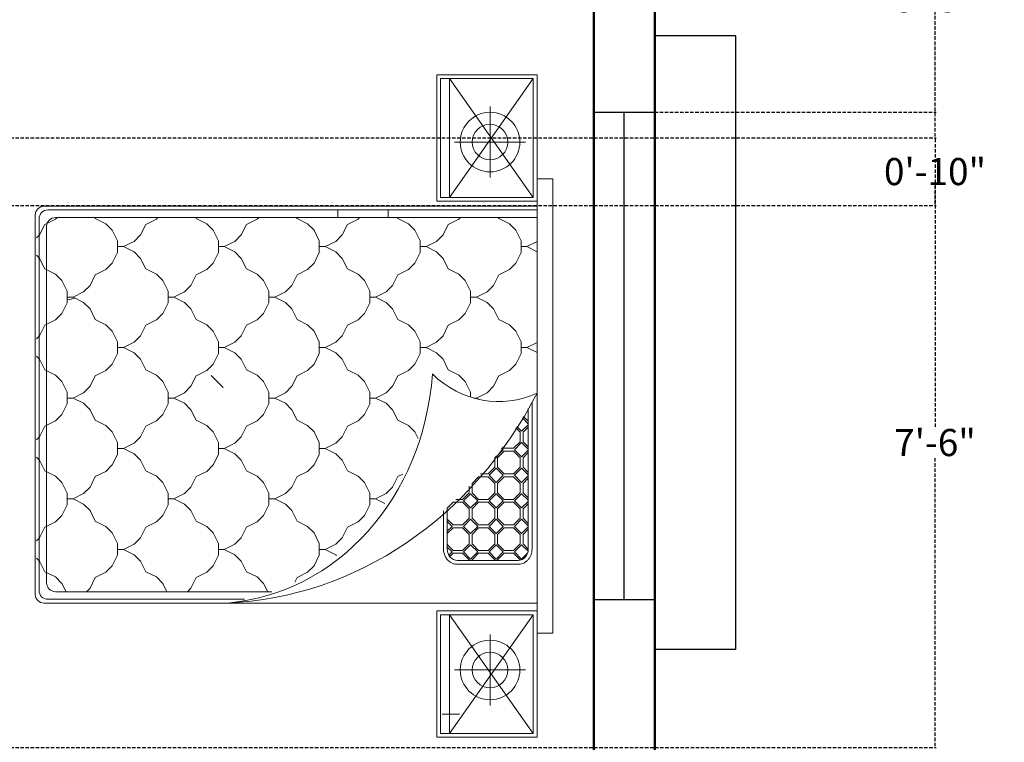
# Model space of a CAD drawing. Units: inches. Extents: x 513 to 1142, y 396 to 927.
# Tile 13 of 31: x 996 to 1142, y 507 to 614. Entities that reach past the tile are written whole.
import ezdxf

# ---------------------------------------------------------------- set-up
doc = ezdxf.new("R2010")
doc.units = ezdxf.units.IN
doc.header["$MEASUREMENT"] = 0
doc.linetypes.add('DASHED', pattern=[0.75, 0.5, -0.25])
for name, color, linetype, lineweight in [('A-ANNO-DIMS', 2, 'DASHED', 18), ('A-WALL', 7, 'Continuous', 50), ('furniture', 92, 'Continuous', 18), ('windows', 172, 'Continuous', 25)]:
    doc.layers.add(name, color=color, linetype=linetype, lineweight=lineweight)
doc.styles.get("Standard").update_dxf_attribs({"font": 'arial.ttf'})
doc.dimstyles.get("Standard").update_dxf_attribs({"dimtxt": 4, "dimasz": 0.18, "dimexe": 0.18, "dimexo": 0.0625, "dimgap": 0.09, "dimtad": 0, "dimtih": 1, "dimtoh": 1, "dimdec": 0, "dimrnd": 6, "dimzin": 0, "dimdsep": 46, "dimlunit": 3, "dimtxsty": 'Standard', "dimcen": 0.09, "dimadec": 0, "dimazin": 0, "dimtfac": 1, "dimtdec": 0, "dimtofl": 0, "dimtmove": 0, "dimatfit": 3, "dimfxl": 1, "dimtolj": 1, "dimtzin": 0, "dimarcsym": 0})

# ---------------------------------------------------------------- blocks, each defined once
blk = doc.blocks.new('A$C029D5C69')
for p, q in [((0.4164, 2.0693), (0.4164, 2.0066)), ((2.2315, 2.0693), (0.4164, 2.0693)), ((2.2315, 2.0066), (2.2315, 2.0693)), ((2.1114, 2.0087), (2.1114, 0.0351)), ((0, 1.606), (0, 2.0066)), ((0, 2.0066), (0.505, 2.0066)), ((0.0151, 1.6211), (0.0151, 1.9915)), ((0.0151, 1.9915), (0.4899, 1.9915)), ((0.4164, 2.0066), (2.2315, 2.0066)), ((0.4899, 1.9915), (0.4899, 1.6211)), ((0.505, 2.0066), (0.505, 1.606)), ((0.5252, 0.0351), (0.5252, 2.0066)), ((0.5403, 0.0502), (0.5403, 2.0066)), ((0.5706, 0.0805), (0.5706, 2.0066)), ((0.6869, 1.966), (0.6666, 2.0066)), ((0.7072, 2.0066), (0.6869, 1.966)), ((1.0902, 1.966), (1.0699, 2.0066)), ((1.1106, 2.0066), (1.0902, 1.966)), ((1.8954, 1.9865), (1.3081, 1.9865)), ((1.8954, 1.9713), (1.3339, 1.9713)), ((1.3849, 1.9713), (1.3656, 1.952)), ((1.3945, 1.9713), (1.3714, 1.9483)), ((1.4249, 1.945), (1.3986, 1.9713)), ((1.4288, 1.9507), (1.4081, 1.9713)), ((1.487, 1.9713), (1.4664, 1.9507)), ((1.4966, 1.9713), (1.4703, 1.945)), ((1.527, 1.945), (1.5007, 1.9713)), ((1.5309, 1.9507), (1.5102, 1.9713)), ((1.5891, 1.9713), (1.5685, 1.9507)), ((1.5987, 1.9713), (1.5724, 1.945)), ((1.6291, 1.945), (1.6028, 1.9713)), ((1.633, 1.9507), (1.6123, 1.9713)), ((1.6912, 1.9713), (1.6706, 1.9507)), ((1.7008, 1.9713), (1.6745, 1.945)), ((1.7312, 1.945), (1.7049, 1.9713)), ((1.7351, 1.9507), (1.7144, 1.9713)), ((1.7933, 1.9713), (1.7727, 1.9507)), ((1.8029, 1.9713), (1.7766, 1.945)), ((1.8333, 1.945), (1.807, 1.9713)), ((1.8372, 1.9507), (1.8165, 1.9713)), ((1.8954, 1.9713), (1.8748, 1.9507)), ((1.9043, 1.9707), (1.8787, 1.945)), ((1.9354, 1.945), (1.9114, 1.969)), ((2.6479, 2.0066), (2.1429, 2.0066)), ((2.1429, 2.0066), (2.1429, 1.606)), ((2.6328, 1.9915), (2.158, 1.9915)), ((2.158, 1.9915), (2.158, 1.6211)), ((2.6328, 1.6211), (2.6328, 1.9915)), ((2.6479, 1.606), (2.6479, 2.0066)), ((0.2689, 1.9609), (0.2689, 1.6764)), ((0.6634, 1.9425), (0.621, 1.9213)), ((0.6634, 1.9425), (0.621, 1.9213)), ((0.6869, 1.9425), (0.6634, 1.9425)), ((0.6869, 1.9425), (0.6869, 1.966)), ((0.6869, 1.9425), (0.6869, 1.966)), ((0.6869, 1.9425), (0.7104, 1.9425)), ((0.7528, 1.9213), (0.7104, 1.9425)), ((0.7528, 1.9213), (0.7104, 1.9425)), ((1.0668, 1.9425), (1.0244, 1.9213)), ((1.0668, 1.9425), (1.0244, 1.9213)), ((1.0902, 1.9425), (1.0668, 1.9425)), ((1.0902, 1.9425), (1.0902, 1.966)), ((1.0902, 1.9425), (1.0902, 1.966)), ((1.0902, 1.9425), (1.1137, 1.9425)), ((1.1561, 1.9213), (1.1137, 1.9425)), ((1.1561, 1.9213), (1.1137, 1.9425)), ((1.4249, 1.945), (1.4059, 1.926)), ((1.4288, 1.9394), (1.4116, 1.9222)), ((1.4476, 1.9507), (1.4288, 1.9507)), ((1.4288, 1.9393), (1.4476, 1.9393)), ((1.4476, 1.9507), (1.4664, 1.9507)), ((1.4664, 1.9393), (1.4476, 1.9393)), ((1.493, 1.9128), (1.4664, 1.9394)), ((1.4986, 1.9167), (1.4703, 1.945)), ((1.527, 1.945), (1.4986, 1.9167)), ((1.5309, 1.9394), (1.5043, 1.9128)), ((1.5497, 1.9507), (1.5309, 1.9507)), ((1.5309, 1.9393), (1.5497, 1.9393)), ((1.5497, 1.9507), (1.5685, 1.9507)), ((1.5685, 1.9393), (1.5497, 1.9393)), ((1.595, 1.9128), (1.5685, 1.9394)), ((1.6007, 1.9167), (1.5724, 1.945)), ((1.6291, 1.945), (1.6007, 1.9167)), ((1.633, 1.9394), (1.6064, 1.9128)), ((1.6518, 1.9507), (1.633, 1.9507)), ((1.633, 1.9393), (1.6518, 1.9393)), ((1.6518, 1.9507), (1.6706, 1.9507)), ((1.6706, 1.9393), (1.6518, 1.9393)), ((1.6971, 1.9128), (1.6706, 1.9394)), ((1.7028, 1.9167), (1.6745, 1.945)), ((1.7312, 1.945), (1.7028, 1.9167)), ((1.7351, 1.9394), (1.7085, 1.9128)), ((1.7539, 1.9507), (1.7351, 1.9507)), ((1.7351, 1.9393), (1.7539, 1.9393)), ((1.7539, 1.9507), (1.7727, 1.9507)), ((1.7727, 1.9393), (1.7539, 1.9393)), ((1.7992, 1.9128), (1.7727, 1.9394)), ((1.8049, 1.9167), (1.7766, 1.945)), ((1.8333, 1.945), (1.8049, 1.9167)), ((1.8372, 1.9394), (1.8106, 1.9128)), ((1.856, 1.9507), (1.8372, 1.9507)), ((1.8372, 1.9393), (1.856, 1.9393)), ((1.856, 1.9507), (1.8748, 1.9507)), ((1.8748, 1.9393), (1.856, 1.9393)), ((1.9013, 1.9128), (1.8748, 1.9394)), ((1.907, 1.9167), (1.8787, 1.945)), ((1.9354, 1.945), (1.907, 1.9167)), ((1.9393, 1.9394), (1.9127, 1.9128)), ((1.9393, 1.9393), (1.9404, 1.9393)), ((1.9414, 1.688), (1.9414, 1.931)), ((1.9565, 1.688), (1.9565, 1.931)), ((2.379, 1.9609), (2.379, 1.6764)), ((0.5955, 1.8958), (0.5743, 1.8534)), ((0.621, 1.9213), (0.5955, 1.8958)), ((0.7783, 1.8958), (0.7528, 1.9213)), ((0.7995, 1.8534), (0.7783, 1.8958)), ((0.9989, 1.8958), (0.9777, 1.8534)), ((1.0243, 1.9213), (0.9988, 1.8958)), ((1.1816, 1.8958), (1.1561, 1.9213)), ((1.2028, 1.8534), (1.1816, 1.8958)), ((1.493, 1.8752), (1.493, 1.9128)), ((1.5043, 1.8752), (1.5043, 1.9128)), ((1.595, 1.8752), (1.595, 1.9128)), ((1.6064, 1.8752), (1.6064, 1.9128)), ((1.6971, 1.8752), (1.6971, 1.9128)), ((1.7085, 1.8752), (1.7085, 1.9128)), ((1.7992, 1.8752), (1.7992, 1.9128)), ((1.8106, 1.8752), (1.8106, 1.9128)), ((1.9013, 1.8752), (1.9013, 1.9128)), ((1.9127, 1.8752), (1.9127, 1.9128)), ((0.5743, 1.8534), (0.5706, 1.8515)), ((0.5743, 1.8534), (0.5706, 1.8515)), ((0.8419, 1.8322), (0.7995, 1.8534)), ((0.8419, 1.8322), (0.7995, 1.8534)), ((0.9777, 1.8534), (0.9353, 1.8322)), ((0.9777, 1.8534), (0.9353, 1.8322)), ((1.2452, 1.8322), (1.2028, 1.8534)), ((1.2452, 1.8322), (1.2028, 1.8534)), ((1.493, 1.8752), (1.4867, 1.869)), ((1.4986, 1.8713), (1.4922, 1.8648)), ((1.527, 1.8429), (1.4986, 1.8713)), ((1.5309, 1.8486), (1.5043, 1.8752)), ((1.595, 1.8752), (1.5685, 1.8486)), ((1.6007, 1.8713), (1.5724, 1.8429)), ((1.6291, 1.8429), (1.6007, 1.8713)), ((1.633, 1.8486), (1.6064, 1.8752)), ((1.6971, 1.8752), (1.6706, 1.8486)), ((1.7028, 1.8713), (1.6745, 1.8429)), ((1.7312, 1.8429), (1.7028, 1.8713)), ((1.7351, 1.8486), (1.7085, 1.8752)), ((1.7992, 1.8752), (1.7727, 1.8486)), ((1.8049, 1.8713), (1.7766, 1.8429)), ((1.8333, 1.8429), (1.8049, 1.8713)), ((1.8372, 1.8486), (1.8106, 1.8752)), ((1.9013, 1.8752), (1.8748, 1.8486)), ((1.907, 1.8713), (1.8787, 1.8429)), ((1.9354, 1.8429), (1.907, 1.8713)), ((1.9393, 1.8486), (1.9127, 1.8752)), ((0.1267, 1.8186), (0.4111, 1.8186)), ((0.8674, 1.8067), (0.8419, 1.8322)), ((0.9352, 1.8322), (0.9097, 1.8067)), ((1.2707, 1.8067), (1.2452, 1.8322)), ((1.527, 1.8429), (1.5242, 1.8401)), ((1.5309, 1.8373), (1.5295, 1.8359)), ((1.5497, 1.8486), (1.5309, 1.8486)), ((1.5309, 1.8373), (1.5497, 1.8373)), ((1.5497, 1.8486), (1.5685, 1.8486)), ((1.5685, 1.8373), (1.5497, 1.8373)), ((1.595, 1.8107), (1.5685, 1.8373)), ((1.6007, 1.8146), (1.5724, 1.8429)), ((1.6291, 1.8429), (1.6007, 1.8146)), ((1.633, 1.8373), (1.6064, 1.8107)), ((1.6518, 1.8486), (1.633, 1.8486)), ((1.633, 1.8373), (1.6518, 1.8373)), ((1.6518, 1.8486), (1.6706, 1.8486)), ((1.6706, 1.8373), (1.6518, 1.8373)), ((1.6971, 1.8107), (1.6706, 1.8373)), ((1.7028, 1.8146), (1.6745, 1.8429)), ((1.7312, 1.8429), (1.7028, 1.8146)), ((1.7351, 1.8373), (1.7085, 1.8107)), ((1.7539, 1.8486), (1.7351, 1.8486)), ((1.7351, 1.8373), (1.7539, 1.8373)), ((1.7539, 1.8486), (1.7727, 1.8486)), ((1.7727, 1.8373), (1.7539, 1.8373)), ((1.7992, 1.8107), (1.7727, 1.8373)), ((1.8049, 1.8146), (1.7766, 1.8429)), ((1.8333, 1.8429), (1.8049, 1.8146)), ((1.8372, 1.8373), (1.8106, 1.8107)), ((1.856, 1.8486), (1.8372, 1.8486)), ((1.8372, 1.8373), (1.856, 1.8373)), ((1.856, 1.8486), (1.8748, 1.8486)), ((1.8748, 1.8373), (1.856, 1.8373)), ((1.9013, 1.8107), (1.8748, 1.8373)), ((1.907, 1.8146), (1.8787, 1.8429)), ((1.9354, 1.8429), (1.907, 1.8146)), ((1.9393, 1.8373), (1.9127, 1.8107)), ((1.9414, 1.8486), (1.9393, 1.8486)), ((1.9393, 1.8373), (1.9414, 1.8373)), ((2.2367, 1.8186), (2.5212, 1.8186)), ((0.8886, 1.7643), (0.8674, 1.8067)), ((0.9098, 1.8067), (0.8886, 1.7643)), ((1.2919, 1.7643), (1.2707, 1.8067)), ((1.2981, 1.7768), (1.2919, 1.7643)), ((1.595, 1.7806), (1.595, 1.8107)), ((1.6064, 1.7731), (1.6064, 1.8107)), ((1.633, 1.7465), (1.6064, 1.7731)), ((1.6971, 1.7731), (1.6706, 1.7465)), ((1.6971, 1.7731), (1.6971, 1.8107)), ((1.7085, 1.7731), (1.7085, 1.8107)), ((1.7351, 1.7465), (1.7085, 1.7731)), ((1.7992, 1.7731), (1.7727, 1.7465)), ((1.7992, 1.7731), (1.7992, 1.8107)), ((1.8106, 1.7731), (1.8106, 1.8107)), ((1.8372, 1.7465), (1.8106, 1.7731)), ((1.9013, 1.7731), (1.8748, 1.7465)), ((1.9013, 1.7731), (1.9013, 1.8107)), ((1.9127, 1.7731), (1.9127, 1.8107)), ((1.9393, 1.7465), (1.9127, 1.7731)), ((0.8651, 1.7408), (0.8227, 1.7196)), ((0.8651, 1.7408), (0.8227, 1.7196)), ((0.912, 1.7408), (0.8651, 1.7408)), ((0.8886, 1.7408), (0.8886, 1.7643)), ((0.9544, 1.7196), (0.912, 1.7408)), ((0.9544, 1.7196), (0.912, 1.7408)), ((1.2684, 1.7408), (1.226, 1.7196)), ((1.2684, 1.7408), (1.226, 1.7196)), ((1.2885, 1.7408), (1.2684, 1.7408)), ((1.2919, 1.7519), (1.2919, 1.7643)), ((1.6518, 1.7465), (1.633, 1.7465)), ((1.6443, 1.7352), (1.6518, 1.7352)), ((1.6518, 1.7465), (1.6706, 1.7465)), ((1.6706, 1.7352), (1.6518, 1.7352)), ((1.6971, 1.7086), (1.6706, 1.7352)), ((1.7028, 1.7692), (1.6745, 1.7408)), ((1.7028, 1.7125), (1.6745, 1.7408)), ((1.7312, 1.7408), (1.7028, 1.7692)), ((1.7312, 1.7408), (1.7028, 1.7125)), ((1.7351, 1.7352), (1.7085, 1.7086)), ((1.7539, 1.7465), (1.7351, 1.7465)), ((1.7351, 1.7352), (1.7539, 1.7352)), ((1.7539, 1.7465), (1.7727, 1.7465)), ((1.7727, 1.7352), (1.7539, 1.7352)), ((1.7992, 1.7086), (1.7727, 1.7352)), ((1.8049, 1.7692), (1.7766, 1.7408)), ((1.8049, 1.7125), (1.7766, 1.7408)), ((1.8333, 1.7408), (1.8049, 1.7692)), ((1.8333, 1.7408), (1.8049, 1.7125)), ((1.8372, 1.7352), (1.8106, 1.7086)), ((1.856, 1.7465), (1.8372, 1.7465)), ((1.8372, 1.7352), (1.856, 1.7352)), ((1.856, 1.7465), (1.8748, 1.7465)), ((1.8748, 1.7352), (1.856, 1.7352)), ((1.9013, 1.7086), (1.8748, 1.7352)), ((1.907, 1.7692), (1.8787, 1.7408)), ((1.907, 1.7125), (1.8787, 1.7408)), ((1.9354, 1.7408), (1.907, 1.7692)), ((1.9354, 1.7408), (1.907, 1.7125)), ((1.9393, 1.7352), (1.9127, 1.7086)), ((1.9414, 1.7465), (1.9393, 1.7465)), ((1.9393, 1.7352), (1.9414, 1.7352)), ((0.5766, 1.6941), (0.5706, 1.7002)), ((0.5978, 1.6517), (0.5766, 1.6941)), ((0.7972, 1.6941), (0.776, 1.6517)), ((0.8227, 1.7196), (0.7972, 1.6941)), ((0.98, 1.6941), (0.9545, 1.7196)), ((1.0011, 1.6517), (0.9799, 1.6941)), ((1.2005, 1.6941), (1.1793, 1.6517)), ((1.226, 1.7196), (1.2005, 1.6941)), ((1.6971, 1.682), (1.6971, 1.7086)), ((1.7085, 1.671), (1.7085, 1.7086)), ((1.7992, 1.671), (1.7992, 1.7086)), ((1.8106, 1.671), (1.8106, 1.7086)), ((1.9013, 1.671), (1.9013, 1.7086)), ((1.9127, 1.671), (1.9127, 1.7086)), ((2.5551, 1.6275), (2.5551, 1.696)), ((1.7318, 1.6477), (1.7085, 1.671)), ((1.7992, 1.671), (1.7759, 1.6477)), ((1.8049, 1.6671), (1.7855, 1.6477)), ((1.8244, 1.6477), (1.8049, 1.6671)), ((1.8339, 1.6477), (1.8106, 1.671)), ((1.9013, 1.671), (1.878, 1.6477)), ((1.907, 1.6671), (1.8876, 1.6477)), ((1.9202, 1.6539), (1.907, 1.6671)), ((1.926, 1.6577), (1.9127, 1.671)), ((0.4899, 1.6211), (0.0151, 1.6211)), ((0.6402, 1.6305), (0.5978, 1.6517)), ((0.6402, 1.6305), (0.5978, 1.6517)), ((0.6657, 1.605), (0.6402, 1.6305)), ((0.7336, 1.6305), (0.7081, 1.605)), ((0.776, 1.6517), (0.7336, 1.6305)), ((0.776, 1.6517), (0.7336, 1.6305)), ((1.0435, 1.6305), (1.0011, 1.6517)), ((1.0435, 1.6305), (1.0011, 1.6517)), ((1.0691, 1.605), (1.0436, 1.6305)), ((1.1369, 1.6305), (1.1114, 1.605)), ((1.1793, 1.6517), (1.1369, 1.6305)), ((1.1793, 1.6517), (1.1369, 1.6305)), ((1.8961, 1.6477), (1.7289, 1.6477)), ((1.8961, 1.6325), (1.7422, 1.6325)), ((2.158, 1.6211), (2.6328, 1.6211)), ((0.505, 1.606), (0, 1.606)), ((0.6869, 1.5626), (0.6657, 1.605)), ((0.7081, 1.605), (0.6869, 1.5626)), ((1.0902, 1.5626), (1.069, 1.605)), ((1.1114, 1.605), (1.0902, 1.5626)), ((2.1429, 1.606), (2.6479, 1.606)), ((0.6634, 1.5391), (0.621, 1.5179)), ((0.6634, 1.5391), (0.621, 1.5179)), ((0.6869, 1.5392), (0.6634, 1.5392)), ((0.6869, 1.5392), (0.6869, 1.5626)), ((0.6869, 1.5392), (0.6869, 1.5626)), ((0.6869, 1.5392), (0.7104, 1.5392)), ((0.7528, 1.5179), (0.7104, 1.5391)), ((0.7528, 1.5179), (0.7104, 1.5391)), ((1.0668, 1.5391), (1.0244, 1.5179)), ((1.0668, 1.5391), (1.0244, 1.5179)), ((1.0902, 1.5392), (1.0668, 1.5392)), ((1.0902, 1.5392), (1.0902, 1.5626)), ((1.0902, 1.5392), (1.0902, 1.5626)), ((1.0902, 1.5392), (1.1137, 1.5392)), ((1.1561, 1.5179), (1.1137, 1.5391)), ((1.1561, 1.5179), (1.1137, 1.5391)), ((0.621, 1.5179), (0.5955, 1.4924)), ((0.7783, 1.4924), (0.7528, 1.5179)), ((1.0243, 1.5179), (0.9988, 1.4924)), ((1.1816, 1.4924), (1.1561, 1.5179)), ((1.4277, 1.5179), (1.4022, 1.4924)), ((1.4534, 1.5308), (1.4277, 1.5179)), ((1.4534, 1.5308), (1.4277, 1.5179)), ((0.5955, 1.4925), (0.5743, 1.4501)), ((0.7995, 1.4501), (0.7783, 1.4925)), ((0.9989, 1.4925), (0.9777, 1.4501)), ((1.2028, 1.4501), (1.1816, 1.4925)), ((1.4022, 1.4925), (1.381, 1.4501)), ((1.6062, 1.4501), (1.5966, 1.4692)), ((0.5743, 1.45), (0.5706, 1.4481)), ((0.5743, 1.45), (0.5706, 1.4481)), ((0.8419, 1.4288), (0.7995, 1.45)), ((0.8419, 1.4288), (0.7995, 1.45)), ((0.8674, 1.4033), (0.8419, 1.4288)), ((0.9352, 1.4288), (0.9097, 1.4033)), ((0.9777, 1.45), (0.9353, 1.4288)), ((0.9777, 1.45), (0.9353, 1.4288)), ((1.2452, 1.4288), (1.2028, 1.45)), ((1.2452, 1.4288), (1.2028, 1.45)), ((1.2707, 1.4033), (1.2452, 1.4288)), ((1.3386, 1.4288), (1.3131, 1.4033)), ((1.381, 1.45), (1.3386, 1.4288)), ((1.381, 1.45), (1.3386, 1.4288)), ((1.6486, 1.4288), (1.6062, 1.45)), ((1.6486, 1.4288), (1.6062, 1.45)), ((1.6741, 1.4033), (1.6486, 1.4288)), ((0.5403, 1.4117), (0.5706, 1.4117)), ((0.8886, 1.361), (0.8674, 1.4034)), ((0.9098, 1.4034), (0.8886, 1.361)), ((1.2919, 1.361), (1.2707, 1.4034)), ((1.3131, 1.4034), (1.2919, 1.361)), ((1.6953, 1.361), (1.6741, 1.4034)), ((1.714, 1.3984), (1.6953, 1.361)), ((0.8886, 1.3375), (0.8886, 1.3609)), ((1.2919, 1.3375), (1.2919, 1.3609)), ((1.6953, 1.3375), (1.6953, 1.3609)), ((0.8227, 1.3163), (0.7972, 1.2908)), ((0.8651, 1.3374), (0.8227, 1.3162)), ((0.8651, 1.3374), (0.8227, 1.3162)), ((0.912, 1.3375), (0.8651, 1.3375)), ((0.9544, 1.3162), (0.912, 1.3374)), ((0.9544, 1.3162), (0.912, 1.3374)), ((0.98, 1.2908), (0.9545, 1.3163)), ((1.226, 1.3163), (1.2005, 1.2908)), ((1.2684, 1.3374), (1.226, 1.3162)), ((1.2684, 1.3374), (1.226, 1.3162)), ((1.3154, 1.3375), (1.2684, 1.3375)), ((1.3578, 1.3162), (1.3154, 1.3374)), ((1.3578, 1.3162), (1.3154, 1.3374)), ((1.3833, 1.2908), (1.3578, 1.3163)), ((1.6294, 1.3163), (1.6039, 1.2908)), ((1.6718, 1.3374), (1.6294, 1.3162)), ((1.6718, 1.3374), (1.6294, 1.3162)), ((1.7187, 1.3375), (1.6718, 1.3375)), ((1.7611, 1.3162), (1.7187, 1.3374)), ((1.7611, 1.3162), (1.7187, 1.3374)), ((1.7867, 1.2908), (1.7611, 1.3163)), ((0.5766, 1.2908), (0.5706, 1.2968)), ((0.5978, 1.2484), (0.5766, 1.2908)), ((0.7972, 1.2908), (0.776, 1.2484)), ((1.0011, 1.2484), (0.9799, 1.2908)), ((1.2005, 1.2908), (1.1793, 1.2484)), ((1.4045, 1.2484), (1.3833, 1.2908)), ((1.6039, 1.2908), (1.5827, 1.2484)), ((1.8078, 1.2484), (1.7866, 1.2908)), ((0.6402, 1.2271), (0.5978, 1.2483)), ((0.6402, 1.2271), (0.5978, 1.2483)), ((0.6657, 1.2017), (0.6402, 1.2272)), ((0.7336, 1.2272), (0.7081, 1.2017)), ((0.776, 1.2483), (0.7336, 1.2271)), ((0.776, 1.2483), (0.7336, 1.2271)), ((1.0435, 1.2271), (1.0011, 1.2483)), ((1.0435, 1.2271), (1.0011, 1.2483)), ((1.0691, 1.2017), (1.0436, 1.2272)), ((1.1369, 1.2272), (1.1114, 1.2017)), ((1.1793, 1.2483), (1.1369, 1.2271)), ((1.1793, 1.2483), (1.1369, 1.2271)), ((1.4469, 1.2271), (1.4045, 1.2483)), ((1.4469, 1.2271), (1.4045, 1.2483)), ((1.4724, 1.2017), (1.4469, 1.2272)), ((1.5403, 1.2272), (1.5148, 1.2017)), ((1.5827, 1.2483), (1.5403, 1.2271)), ((1.5827, 1.2483), (1.5403, 1.2271)), ((1.8502, 1.2271), (1.8078, 1.2483)), ((1.8502, 1.2271), (1.8078, 1.2483)), ((1.8758, 1.2017), (1.8503, 1.2272)), ((0.5403, 1.21), (0.5706, 1.21)), ((0.6869, 1.1593), (0.6657, 1.2017)), ((0.7081, 1.2017), (0.6869, 1.1593)), ((1.0902, 1.1593), (1.069, 1.2017)), ((1.1114, 1.2017), (1.0902, 1.1593)), ((1.4936, 1.1593), (1.4724, 1.2017)), ((1.5148, 1.2017), (1.4936, 1.1593)), ((1.8969, 1.1593), (1.8757, 1.2017)), ((1.9181, 1.2017), (1.8969, 1.1593)), ((1.9215, 1.2051), (1.9181, 1.2017)), ((0.6869, 1.1358), (0.6869, 1.1593)), ((0.6869, 1.1358), (0.6869, 1.1593)), ((1.0902, 1.1358), (1.0902, 1.1593)), ((1.0902, 1.1358), (1.0902, 1.1593)), ((1.4936, 1.1358), (1.4936, 1.1593)), ((1.4936, 1.1358), (1.4936, 1.1593)), ((1.8969, 1.1358), (1.8969, 1.1593)), ((1.8969, 1.1358), (1.8969, 1.1593)), ((0.621, 1.1146), (0.5955, 1.0891)), ((0.6634, 1.1358), (0.621, 1.1146)), ((0.6634, 1.1358), (0.621, 1.1146)), ((0.6869, 1.1358), (0.6634, 1.1358)), ((0.6869, 1.1358), (0.7104, 1.1358)), ((0.7528, 1.1146), (0.7104, 1.1358)), ((0.7528, 1.1146), (0.7104, 1.1358)), ((0.7783, 1.0891), (0.7528, 1.1146)), ((1.0243, 1.1146), (0.9988, 1.0891)), ((1.0668, 1.1358), (1.0244, 1.1146)), ((1.0668, 1.1358), (1.0244, 1.1146)), ((1.0902, 1.1358), (1.0668, 1.1358)), ((1.0902, 1.1358), (1.1137, 1.1358)), ((1.1561, 1.1146), (1.1137, 1.1358)), ((1.1561, 1.1146), (1.1137, 1.1358)), ((1.1816, 1.0891), (1.1561, 1.1146)), ((1.4277, 1.1146), (1.4022, 1.0891)), ((1.4701, 1.1358), (1.4277, 1.1146)), ((1.4701, 1.1358), (1.4277, 1.1146)), ((1.4936, 1.1358), (1.4701, 1.1358)), ((1.4936, 1.1358), (1.5171, 1.1358)), ((1.5595, 1.1146), (1.5171, 1.1358)), ((1.5595, 1.1146), (1.5171, 1.1358)), ((1.585, 1.0891), (1.5595, 1.1146)), ((1.831, 1.1146), (1.8055, 1.0891)), ((1.8735, 1.1358), (1.8311, 1.1146)), ((1.8735, 1.1358), (1.8311, 1.1146)), ((1.8969, 1.1358), (1.8735, 1.1358)), ((1.8969, 1.1358), (1.9204, 1.1358)), ((1.9628, 1.1146), (1.9204, 1.1358)), ((1.9628, 1.1146), (1.9204, 1.1358)), ((1.9883, 1.0891), (1.9628, 1.1146)), ((0.5955, 1.0891), (0.5743, 1.0467)), ((0.7995, 1.0467), (0.7783, 1.0891)), ((0.9989, 1.0891), (0.9777, 1.0467)), ((1.2028, 1.0467), (1.1816, 1.0891)), ((1.4022, 1.0891), (1.381, 1.0467)), ((1.6062, 1.0467), (1.585, 1.0891)), ((1.8056, 1.0891), (1.7844, 1.0467)), ((2.0095, 1.0467), (1.9883, 1.0891)), ((0.5743, 1.0467), (0.5706, 1.0448)), ((0.5743, 1.0467), (0.5706, 1.0448)), ((0.8419, 1.0255), (0.7995, 1.0467)), ((0.8419, 1.0255), (0.7995, 1.0467)), ((0.8674, 1), (0.8419, 1.0255)), ((0.9352, 1.0255), (0.9097, 1)), ((0.9777, 1.0467), (0.9353, 1.0255)), ((0.9777, 1.0467), (0.9353, 1.0255)), ((1.2452, 1.0255), (1.2028, 1.0467)), ((1.2452, 1.0255), (1.2028, 1.0467)), ((1.2707, 1), (1.2452, 1.0255)), ((1.3386, 1.0255), (1.3131, 1)), ((1.381, 1.0467), (1.3386, 1.0255)), ((1.381, 1.0467), (1.3386, 1.0255)), ((1.6486, 1.0255), (1.6062, 1.0467)), ((1.6486, 1.0255), (1.6062, 1.0467)), ((1.6741, 1), (1.6486, 1.0255)), ((1.7419, 1.0255), (1.7164, 1)), ((1.7844, 1.0467), (1.742, 1.0255)), ((1.7844, 1.0467), (1.742, 1.0255)), ((2.0276, 1.0376), (2.0095, 1.0467)), ((2.0276, 1.0376), (2.0095, 1.0467)), ((0.8886, 0.9576), (0.8674, 1)), ((0.9098, 1), (0.8886, 0.9576)), ((1.2919, 0.9576), (1.2707, 1)), ((1.3131, 1), (1.2919, 0.9576)), ((1.6953, 0.9576), (1.6741, 1)), ((1.7165, 1), (1.6953, 0.9576)), ((0.8886, 0.9341), (0.8886, 0.9576)), ((1.2919, 0.9341), (1.2919, 0.9576)), ((1.6953, 0.9341), (1.6953, 0.9576)), ((2.066, 0.9457), (2.066, 0.0805)), ((0.8227, 0.9129), (0.7972, 0.8874)), ((0.8651, 0.9341), (0.8227, 0.9129)), ((0.8651, 0.9341), (0.8227, 0.9129)), ((0.912, 0.9341), (0.8651, 0.9341)), ((0.9544, 0.9129), (0.912, 0.9341)), ((0.9544, 0.9129), (0.912, 0.9341)), ((0.98, 0.8874), (0.9545, 0.9129)), ((1.226, 0.9129), (1.2005, 0.8874)), ((1.2684, 0.9341), (1.226, 0.9129)), ((1.2684, 0.9341), (1.226, 0.9129)), ((1.3154, 0.9341), (1.2684, 0.9341)), ((1.3578, 0.9129), (1.3154, 0.9341)), ((1.3578, 0.9129), (1.3154, 0.9341)), ((1.3833, 0.8874), (1.3578, 0.9129)), ((1.6294, 0.9129), (1.6039, 0.8874)), ((1.6718, 0.9341), (1.6294, 0.9129)), ((1.6718, 0.9341), (1.6294, 0.9129)), ((1.7187, 0.9341), (1.6718, 0.9341)), ((1.7611, 0.9129), (1.7187, 0.9341)), ((1.7611, 0.9129), (1.7187, 0.9341)), ((1.7867, 0.8874), (1.7611, 0.9129)), ((2.0327, 0.9129), (2.0072, 0.8874)), ((2.066, 0.9295), (2.0327, 0.9129)), ((2.066, 0.9295), (2.0327, 0.9129)), ((0.5766, 0.8874), (0.5706, 0.8935)), ((0.5978, 0.845), (0.5766, 0.8874)), ((0.7972, 0.8874), (0.776, 0.845)), ((1.0011, 0.845), (0.9799, 0.8874)), ((1.2005, 0.8874), (1.1793, 0.845)), ((1.4045, 0.845), (1.3833, 0.8874)), ((1.6039, 0.8874), (1.5827, 0.845)), ((1.8078, 0.845), (1.7866, 0.8874)), ((2.0072, 0.8874), (1.986, 0.845)), ((0.6402, 0.8238), (0.5978, 0.845)), ((0.6402, 0.8238), (0.5978, 0.845)), ((0.776, 0.845), (0.7336, 0.8238)), ((0.776, 0.845), (0.7336, 0.8238)), ((1.0435, 0.8238), (1.0011, 0.845)), ((1.0435, 0.8238), (1.0011, 0.845)), ((1.1793, 0.845), (1.1369, 0.8238)), ((1.1793, 0.845), (1.1369, 0.8238)), ((1.4469, 0.8238), (1.4045, 0.845)), ((1.4469, 0.8238), (1.4045, 0.845)), ((1.5827, 0.845), (1.5403, 0.8238)), ((1.5827, 0.845), (1.5403, 0.8238)), ((1.8502, 0.8238), (1.8078, 0.845)), ((1.8502, 0.8238), (1.8078, 0.845)), ((1.986, 0.845), (1.9436, 0.8238)), ((1.986, 0.845), (1.9436, 0.8238)), ((2.0962, 0.8369), (2.0962, 0.0502)), ((0.6657, 0.7983), (0.6402, 0.8238)), ((0.6869, 0.7559), (0.6657, 0.7983)), ((0.7081, 0.7983), (0.6869, 0.7559)), ((0.7336, 0.8238), (0.7081, 0.7983)), ((1.0691, 0.7983), (1.0436, 0.8238)), ((1.0902, 0.7559), (1.069, 0.7983)), ((1.1114, 0.7983), (1.0902, 0.7559)), ((1.1369, 0.8238), (1.1114, 0.7983)), ((1.4724, 0.7983), (1.4469, 0.8238)), ((1.4936, 0.7559), (1.4724, 0.7983)), ((1.5148, 0.7983), (1.4936, 0.7559)), ((1.5403, 0.8238), (1.5148, 0.7983)), ((1.8758, 0.7983), (1.8503, 0.8238)), ((1.8969, 0.7559), (1.8757, 0.7983)), ((1.9181, 0.7983), (1.8969, 0.7559)), ((1.9436, 0.8238), (1.9181, 0.7983)), ((0.6869, 0.7325), (0.6869, 0.7559)), ((0.6869, 0.7325), (0.6869, 0.7559)), ((1.0902, 0.7325), (1.0902, 0.7559)), ((1.0902, 0.7325), (1.0902, 0.7559)), ((1.2024, 0.7028), (1.2503, 0.7507)), ((1.4936, 0.7325), (1.4936, 0.7559)), ((1.4936, 0.7325), (1.4936, 0.7559)), ((1.8969, 0.7325), (1.8969, 0.7559)), ((1.8969, 0.7325), (1.8969, 0.7559)), ((0.621, 0.7113), (0.5955, 0.6858)), ((0.6634, 0.7324), (0.621, 0.7112)), ((0.6634, 0.7324), (0.621, 0.7112)), ((0.6869, 0.7325), (0.6634, 0.7325)), ((0.6869, 0.7325), (0.7104, 0.7325)), ((0.7528, 0.7112), (0.7104, 0.7324)), ((0.7528, 0.7112), (0.7104, 0.7324)), ((0.7783, 0.6858), (0.7528, 0.7113)), ((1.0243, 0.7113), (0.9988, 0.6858)), ((1.0668, 0.7324), (1.0244, 0.7112)), ((1.0668, 0.7324), (1.0244, 0.7112)), ((1.0902, 0.7325), (1.0668, 0.7325)), ((1.0902, 0.7325), (1.1137, 0.7325)), ((1.1561, 0.7112), (1.1137, 0.7324)), ((1.1561, 0.7112), (1.1137, 0.7324)), ((1.1816, 0.6858), (1.1561, 0.7113)), ((1.4277, 0.7113), (1.4022, 0.6858)), ((1.4701, 0.7324), (1.4277, 0.7112)), ((1.4701, 0.7324), (1.4277, 0.7112)), ((1.4936, 0.7325), (1.4701, 0.7325)), ((1.4936, 0.7325), (1.5171, 0.7325)), ((1.5595, 0.7112), (1.5171, 0.7324)), ((1.5595, 0.7112), (1.5171, 0.7324)), ((1.585, 0.6858), (1.5595, 0.7113)), ((1.831, 0.7113), (1.8055, 0.6858)), ((1.8735, 0.7324), (1.8311, 0.7112)), ((1.8735, 0.7324), (1.8311, 0.7112)), ((1.8969, 0.7325), (1.8735, 0.7325)), ((1.8969, 0.7325), (1.9204, 0.7325)), ((1.9628, 0.7112), (1.9204, 0.7324)), ((1.9628, 0.7112), (1.9204, 0.7324)), ((1.9883, 0.6858), (1.9628, 0.7113)), ((0.5955, 0.6858), (0.5743, 0.6434)), ((0.7995, 0.6434), (0.7783, 0.6858)), ((0.9989, 0.6858), (0.9777, 0.6434)), ((1.2028, 0.6434), (1.1816, 0.6858)), ((1.4022, 0.6858), (1.381, 0.6434)), ((1.6062, 0.6434), (1.585, 0.6858)), ((1.8056, 0.6858), (1.7844, 0.6434)), ((2.0095, 0.6434), (1.9883, 0.6858)), ((0.5743, 0.6433), (0.5706, 0.6414)), ((0.5743, 0.6433), (0.5706, 0.6414)), ((0.8419, 0.6221), (0.7995, 0.6433)), ((0.8419, 0.6221), (0.7995, 0.6433)), ((0.9777, 0.6433), (0.9353, 0.6221)), ((0.9777, 0.6433), (0.9353, 0.6221)), ((1.2452, 0.6221), (1.2028, 0.6433)), ((1.2452, 0.6221), (1.2028, 0.6433)), ((1.381, 0.6433), (1.3386, 0.6221)), ((1.381, 0.6433), (1.3386, 0.6221)), ((1.6486, 0.6221), (1.6062, 0.6433)), ((1.6486, 0.6221), (1.6062, 0.6433)), ((1.7844, 0.6433), (1.742, 0.6221)), ((1.7844, 0.6433), (1.742, 0.6221)), ((2.0519, 0.6221), (2.0095, 0.6433)), ((2.0519, 0.6221), (2.0095, 0.6433)), ((0.8674, 0.5967), (0.8419, 0.6222)), ((0.8886, 0.5543), (0.8674, 0.5967)), ((0.9098, 0.5967), (0.8886, 0.5543)), ((0.9352, 0.6222), (0.9097, 0.5967)), ((1.2707, 0.5967), (1.2452, 0.6222)), ((1.2919, 0.5543), (1.2707, 0.5967)), ((1.3131, 0.5967), (1.2919, 0.5543)), ((1.3386, 0.6222), (1.3131, 0.5967)), ((1.6741, 0.5967), (1.6486, 0.6222)), ((1.6953, 0.5543), (1.6741, 0.5967)), ((1.7165, 0.5967), (1.6953, 0.5543)), ((1.7419, 0.6222), (1.7164, 0.5967)), ((2.066, 0.6081), (2.0519, 0.6222)), ((0.8886, 0.5308), (0.8886, 0.5543)), ((1.2919, 0.5308), (1.2919, 0.5543)), ((1.6953, 0.5308), (1.6953, 0.5543)), ((0.8651, 0.5308), (0.8227, 0.5096)), ((0.8651, 0.5308), (0.8227, 0.5096)), ((0.912, 0.5308), (0.8651, 0.5308)), ((0.9544, 0.5096), (0.912, 0.5308)), ((0.9544, 0.5096), (0.912, 0.5308)), ((1.2684, 0.5308), (1.226, 0.5096)), ((1.2684, 0.5308), (1.226, 0.5096)), ((1.3154, 0.5308), (1.2684, 0.5308)), ((1.3578, 0.5096), (1.3154, 0.5308)), ((1.3578, 0.5096), (1.3154, 0.5308)), ((1.6718, 0.5308), (1.6294, 0.5096)), ((1.6718, 0.5308), (1.6294, 0.5096)), ((1.7187, 0.5308), (1.6718, 0.5308)), ((1.7611, 0.5096), (1.7187, 0.5308)), ((1.7611, 0.5096), (1.7187, 0.5308)), ((2.066, 0.5262), (2.0327, 0.5096)), ((2.066, 0.5262), (2.0327, 0.5096)), ((0.5766, 0.4841), (0.5706, 0.4901)), ((0.5978, 0.4417), (0.5766, 0.4841)), ((0.7972, 0.4841), (0.776, 0.4417)), ((0.8227, 0.5096), (0.7972, 0.4841)), ((0.98, 0.4841), (0.9545, 0.5096)), ((1.0011, 0.4417), (0.9799, 0.4841)), ((1.2005, 0.4841), (1.1793, 0.4417)), ((1.226, 0.5096), (1.2005, 0.4841)), ((1.3833, 0.4841), (1.3578, 0.5096)), ((1.4045, 0.4417), (1.3833, 0.4841)), ((1.6039, 0.4841), (1.5827, 0.4417)), ((1.6294, 0.5096), (1.6039, 0.4841)), ((1.7867, 0.4841), (1.7611, 0.5096)), ((1.8078, 0.4417), (1.7866, 0.4841)), ((2.0072, 0.4841), (1.986, 0.4417)), ((2.0327, 0.5096), (2.0072, 0.4841)), ((0.6402, 0.4205), (0.5978, 0.4417)), ((0.6402, 0.4205), (0.5978, 0.4417)), ((0.776, 0.4417), (0.7336, 0.4205)), ((0.776, 0.4417), (0.7336, 0.4205)), ((1.0435, 0.4205), (1.0011, 0.4417)), ((1.0435, 0.4205), (1.0011, 0.4417)), ((1.1793, 0.4417), (1.1369, 0.4205)), ((1.1793, 0.4417), (1.1369, 0.4205)), ((1.4469, 0.4205), (1.4045, 0.4417)), ((1.4469, 0.4205), (1.4045, 0.4417)), ((1.5827, 0.4417), (1.5403, 0.4205)), ((1.5827, 0.4417), (1.5403, 0.4205)), ((1.8502, 0.4205), (1.8078, 0.4417)), ((1.8502, 0.4205), (1.8078, 0.4417)), ((1.986, 0.4417), (1.9436, 0.4205)), ((1.986, 0.4417), (1.9436, 0.4205)), ((0.6657, 0.395), (0.6402, 0.4205)), ((0.6869, 0.3526), (0.6657, 0.395)), ((0.7081, 0.395), (0.6869, 0.3526)), ((0.7336, 0.4205), (0.7081, 0.395)), ((1.0691, 0.395), (1.0436, 0.4205)), ((1.0902, 0.3526), (1.069, 0.395)), ((1.1114, 0.395), (1.0902, 0.3526)), ((1.1369, 0.4205), (1.1114, 0.395)), ((1.4724, 0.395), (1.4469, 0.4205)), ((1.4936, 0.3526), (1.4724, 0.395)), ((1.5148, 0.395), (1.4936, 0.3526)), ((1.5403, 0.4205), (1.5148, 0.395)), ((1.8758, 0.395), (1.8503, 0.4205)), ((1.8969, 0.3526), (1.8757, 0.395)), ((1.9181, 0.395), (1.8969, 0.3526)), ((1.9436, 0.4205), (1.9181, 0.395)), ((0.6634, 0.3291), (0.621, 0.3079)), ((0.6634, 0.3291), (0.621, 0.3079)), ((0.6869, 0.3291), (0.6634, 0.3291)), ((0.6869, 0.3291), (0.6869, 0.3526)), ((0.6869, 0.3291), (0.6869, 0.3526)), ((0.6869, 0.3291), (0.7104, 0.3291)), ((0.7528, 0.3079), (0.7104, 0.3291)), ((0.7528, 0.3079), (0.7104, 0.3291)), ((1.0668, 0.3291), (1.0244, 0.3079)), ((1.0668, 0.3291), (1.0244, 0.3079)), ((1.0902, 0.3291), (1.0668, 0.3291)), ((1.0902, 0.3291), (1.0902, 0.3526)), ((1.0902, 0.3291), (1.0902, 0.3526)), ((1.0902, 0.3291), (1.1137, 0.3291)), ((1.1561, 0.3079), (1.1137, 0.3291)), ((1.1561, 0.3079), (1.1137, 0.3291)), ((1.4701, 0.3291), (1.4277, 0.3079)), ((1.4701, 0.3291), (1.4277, 0.3079)), ((1.4936, 0.3291), (1.4701, 0.3291)), ((1.4936, 0.3291), (1.4936, 0.3526)), ((1.4936, 0.3291), (1.4936, 0.3526)), ((1.4936, 0.3291), (1.5171, 0.3291)), ((1.5595, 0.3079), (1.5171, 0.3291)), ((1.5595, 0.3079), (1.5171, 0.3291)), ((1.8735, 0.3291), (1.8311, 0.3079)), ((1.8735, 0.3291), (1.8311, 0.3079)), ((1.8969, 0.3291), (1.8735, 0.3291)), ((1.8969, 0.3291), (1.8969, 0.3526)), ((1.8969, 0.3291), (1.8969, 0.3526)), ((1.8969, 0.3291), (1.9204, 0.3291)), ((1.9628, 0.3079), (1.9204, 0.3291)), ((1.9628, 0.3079), (1.9204, 0.3291)), ((0.5955, 0.2824), (0.5743, 0.24)), ((0.621, 0.3079), (0.5955, 0.2824)), ((0.7783, 0.2824), (0.7528, 0.3079)), ((0.7995, 0.24), (0.7783, 0.2824)), ((0.9989, 0.2824), (0.9777, 0.24)), ((1.0243, 0.3079), (0.9988, 0.2824)), ((1.1816, 0.2824), (1.1561, 0.3079)), ((1.2028, 0.24), (1.1816, 0.2824)), ((1.4022, 0.2824), (1.381, 0.24)), ((1.4277, 0.3079), (1.4022, 0.2824)), ((1.585, 0.2824), (1.5595, 0.3079)), ((1.6062, 0.24), (1.585, 0.2824)), ((1.8056, 0.2824), (1.7844, 0.24)), ((1.831, 0.3079), (1.8055, 0.2824)), ((1.9883, 0.2824), (1.9628, 0.3079)), ((2.0095, 0.24), (1.9883, 0.2824)), ((0.5743, 0.24), (0.5706, 0.2381)), ((0.5743, 0.24), (0.5706, 0.2381)), ((0.8419, 0.2188), (0.7995, 0.24)), ((0.8419, 0.2188), (0.7995, 0.24)), ((0.9777, 0.24), (0.9353, 0.2188)), ((0.9777, 0.24), (0.9353, 0.2188)), ((1.2452, 0.2188), (1.2028, 0.24)), ((1.2452, 0.2188), (1.2028, 0.24)), ((1.381, 0.24), (1.3386, 0.2188)), ((1.381, 0.24), (1.3386, 0.2188)), ((1.6486, 0.2188), (1.6062, 0.24)), ((1.6486, 0.2188), (1.6062, 0.24)), ((1.7844, 0.24), (1.742, 0.2188)), ((1.7844, 0.24), (1.742, 0.2188)), ((2.0519, 0.2188), (2.0095, 0.24)), ((2.0519, 0.2188), (2.0095, 0.24)), ((0.8674, 0.1933), (0.8419, 0.2188)), ((0.9352, 0.2188), (0.9097, 0.1933)), ((1.2707, 0.1933), (1.2452, 0.2188)), ((1.3386, 0.2188), (1.3131, 0.1933)), ((1.6741, 0.1933), (1.6486, 0.2188)), ((1.7419, 0.2188), (1.7164, 0.1933)), ((2.066, 0.2047), (2.0519, 0.2188)), ((0.8886, 0.1509), (0.8674, 0.1933)), ((0.9098, 0.1933), (0.8886, 0.1509)), ((1.2919, 0.1509), (1.2707, 0.1933)), ((1.3131, 0.1933), (1.2919, 0.1509)), ((1.6953, 0.1509), (1.6741, 0.1933)), ((1.7165, 0.1933), (1.6953, 0.1509)), ((0.8651, 0.1274), (0.8227, 0.1062)), ((0.8651, 0.1274), (0.8227, 0.1062)), ((0.912, 0.1275), (0.8651, 0.1275)), ((0.8886, 0.1275), (0.8886, 0.1509)), ((0.9544, 0.1062), (0.912, 0.1274)), ((0.9544, 0.1062), (0.912, 0.1274)), ((1.2684, 0.1274), (1.226, 0.1062)), ((1.2684, 0.1274), (1.226, 0.1062)), ((1.3154, 0.1275), (1.2684, 0.1275)), ((1.2919, 0.1275), (1.2919, 0.1509)), ((1.3578, 0.1062), (1.3154, 0.1274)), ((1.3578, 0.1062), (1.3154, 0.1274)), ((1.6718, 0.1274), (1.6294, 0.1062)), ((1.6718, 0.1274), (1.6294, 0.1062)), ((1.7187, 0.1275), (1.6718, 0.1275)), ((1.6953, 0.1275), (1.6953, 0.1509)), ((1.7611, 0.1062), (1.7187, 0.1274)), ((1.7611, 0.1062), (1.7187, 0.1274)), ((2.066, 0.1228), (2.0327, 0.1062)), ((2.066, 0.1228), (2.0327, 0.1062)), ((0.5766, 0.0807), (0.5706, 0.0868)), ((0.5978, 0.0384), (0.5766, 0.0808)), ((0.7972, 0.0808), (0.776, 0.0384)), ((0.8227, 0.1062), (0.7972, 0.0807)), ((0.98, 0.0807), (0.9545, 0.1062)), ((1.0011, 0.0384), (0.9799, 0.0808)), ((1.2005, 0.0808), (1.1793, 0.0384)), ((1.226, 0.1062), (1.2005, 0.0807)), ((1.3833, 0.0807), (1.3578, 0.1062)), ((1.4045, 0.0384), (1.3833, 0.0808)), ((1.6039, 0.0808), (1.5827, 0.0384)), ((1.6294, 0.1062), (1.6039, 0.0807)), ((1.7867, 0.0807), (1.7611, 0.1062)), ((1.8078, 0.0384), (1.7866, 0.0808)), ((2.0072, 0.0808), (1.986, 0.0384)), ((2.0327, 0.1062), (2.0072, 0.0807)), ((2.0309, 0.0454), (0.6056, 0.0454)), ((2.0763, 0), (0.5603, 0)), ((2.0612, 0.0151), (0.5754, 0.0151)), ((0.6402, 0.0171), (0.5978, 0.0383)), ((0.6402, 0.0171), (0.5978, 0.0383)), ((0.6523, 0.005), (0.6402, 0.0171)), ((0.7336, 0.0171), (0.7215, 0.005)), ((0.776, 0.0383), (0.7336, 0.0171)), ((0.776, 0.0383), (0.7336, 0.0171)), ((1.0435, 0.0171), (1.0011, 0.0383)), ((1.0435, 0.0171), (1.0011, 0.0383)), ((1.0557, 0.005), (1.0436, 0.0171)), ((1.1369, 0.0171), (1.1248, 0.005)), ((1.1793, 0.0383), (1.1369, 0.0171)), ((1.1793, 0.0383), (1.1369, 0.0171)), ((1.4469, 0.0171), (1.4045, 0.0383)), ((1.4469, 0.0171), (1.4045, 0.0383)), ((1.459, 0.005), (1.4469, 0.0171)), ((1.5403, 0.0171), (1.5282, 0.005)), ((1.5827, 0.0383), (1.5403, 0.0171)), ((1.5827, 0.0383), (1.5403, 0.0171)), ((1.8502, 0.0171), (1.8078, 0.0383)), ((1.8502, 0.0171), (1.8078, 0.0383)), ((1.8623, 0.005), (1.8503, 0.0171)), ((1.9436, 0.0171), (1.9315, 0.005)), ((1.986, 0.0383), (1.9436, 0.0171)), ((1.986, 0.0383), (1.9436, 0.0171))]:
    blk.add_line(p, q)
at = {"ltscale": 0.005}
for p, q in [((0.4899, 1.6568), (0.0151, 1.9915)), ((0.0151, 1.6568), (0.4899, 1.9915)), ((2.6328, 1.6568), (2.158, 1.9915)), ((2.158, 1.6568), (2.6328, 1.9915)), ((0.0151, 1.6568), (0.4899, 1.6568)), ((2.6328, 1.6568), (2.158, 1.6568))]:
    blk.add_line(p, q, dxfattribs=at)
for centre, radius in [((0.2689, 1.8186), 0.1191), ((2.379, 1.8186), 0.1191), ((0.2689, 1.8186), 0.0711), ((2.379, 1.8186), 0.0711)]:
    blk.add_circle(centre, radius)
for centre, radius, start, end in [((0.2843, 0.0157), 0.6251, 10.2961, 13.2684), ((0.6056, 0.0805), 0.0351, 180, 270), ((2.0309, 0.0805), 0.0351, 270, 0), ((0.5754, 0.0502), 0.0351, 180, 270), ((2.0612, 0.0502), 0.0351, 270, 0), ((0.5603, 0.0351), 0.0351, 180, 270), ((2.0763, 0.0351), 0.0351, 270, 0)]:
    blk.add_arc(centre, radius, start, end)
for centre, major_axis, ratio, start_param, end_param in [((0.8506, 1.8527), (-0.4556, 0), 0.89, 2.430919, 3.53111), ((0.3667, 0.6698), (1.7398, 0.1668), 0.88072, -0.045073, 0.941433), ((1.8961, 1.931), (-0.0453, 0), 0.89, 3.141593, 4.712389), ((1.8961, 1.688), (-0.0453, 0), 0.89, 1.570796, 3.141593), ((1.0874, 0.6748), (1.021, 0.1213), 0.889348, -0.031673, 1.359628)]:
    blk.add_ellipse(centre, major_axis=major_axis, ratio=ratio, start_param=start_param, end_param=end_param)
for points, knots in [([(1.9565, 1.931), (1.9565, 1.9336), (1.9563, 1.9362), (1.9553, 1.9428), (1.9543, 1.9467), (1.9512, 1.9541), (1.9493, 1.9577), (1.9446, 1.9643), (1.942, 1.9674), (1.936, 1.9729), (1.9327, 1.9753), (1.9257, 1.9795), (1.922, 1.9813), (1.9142, 1.9841), (1.9102, 1.9851), (1.9028, 1.9862), (1.8995, 1.9865), (1.8961, 1.9865)], [3.141593, 3.141593, 3.141593, 3.141593, 3.277614, 3.277614, 3.488082, 3.488082, 3.698551, 3.698551, 3.909019, 3.909019, 4.119488, 4.119488, 4.329956, 4.329956, 4.540424, 4.540424, 4.712389, 4.712389, 4.712389, 4.712389]), ([(1.8961, 1.6325), (1.899, 1.6325), (1.9019, 1.6327), (1.9101, 1.6338), (1.9153, 1.6352), (1.9253, 1.6392), (1.93, 1.6418), (1.9385, 1.6481), (1.9423, 1.6519), (1.9481, 1.6594), (1.9503, 1.663), (1.9537, 1.6707), (1.955, 1.6747), (1.9563, 1.6818), (1.9565, 1.6849), (1.9565, 1.688)], [1.570796, 1.570796, 1.570796, 1.570796, 1.718836, 1.718836, 1.993452, 1.993452, 2.268068, 2.268068, 2.542684, 2.542684, 2.761386, 2.761386, 2.980087, 2.980087, 3.141593, 3.141593, 3.141593, 3.141593])]:
    blk.add_open_spline(points, degree=3, knots=knots)
blk = doc.blocks.new('A$C0D3A6DFA')
blk.add_blockref('A$C029D5C69', (0, 0))
blk = doc.blocks.new('WIN-72IN')
blk.add_line((0, 4.45), (72, 4.45))
blk.add_lwpolyline([(72, 9), (72, 0), (0, 0), (0, 9)], close=True)
blk = doc.blocks.new('*D150')
at = {"layer": 'A-ANNO-DIMS', "color": 0, "lineweight": -2, "transparency": 16777216}
for p, q in [((904.06, 596.09), (1131.58, 596.09)), ((1131.4, 595.91), (1131.4, 553.23)), ((1131.4, 506.27), (1131.4, 548.96)), ((904.06, 506.09), (1131.58, 506.09))]:
    blk.add_line(p, q, dxfattribs=at)
at = {"layer": 'A-ANNO-DIMS', "color": 0, "transparency": 16777216}
for points in [[(1131.37, 595.91), (1131.43, 595.91), (1131.4, 596.09)], [(1131.37, 506.27), (1131.43, 506.27), (1131.4, 506.09)]]:
    blk.add_solid(points, dxfattribs=at)
at = {"layer": 'Defpoints', "color": 0, "transparency": 16777216}
for p in [(904, 596.09), (904, 506.09), (1131.4, 506.09)]:
    blk.add_point(p, dxfattribs=at)
at = {"layer": 'A-ANNO-DIMS', "color": 0, "transparency": 16777216, "insert": (1131.4, 551.09), "char_height": 4, "attachment_point": 5}
blk.add_mtext('\\A1;7\'-6"', dxfattribs=at)
blk = doc.blocks.new('*D162')
at = {"layer": 'A-ANNO-DIMS', "color": 0, "lineweight": -2, "transparency": 16777216}
for p, q in [((1081.06, 637.16), (1131.58, 637.16)), ((1131.4, 636.98), (1131.4, 620.68)), ((1131.4, 600.06), (1131.4, 616.36)), ((1080.99, 599.88), (1131.58, 599.88))]:
    blk.add_line(p, q, dxfattribs=at)
at = {"layer": 'A-ANNO-DIMS', "color": 0, "transparency": 16777216}
for points in [[(1131.37, 636.98), (1131.43, 636.98), (1131.4, 637.16)], [(1131.37, 600.06), (1131.43, 600.06), (1131.4, 599.88)]]:
    blk.add_solid(points, dxfattribs=at)
at = {"layer": 'Defpoints', "color": 0, "transparency": 16777216}
for p in [(1081, 637.16), (1080.93, 599.88), (1131.4, 599.88)]:
    blk.add_point(p, dxfattribs=at)
at = {"layer": 'A-ANNO-DIMS', "color": 0, "transparency": 16777216, "insert": (1131.4, 618.52), "char_height": 4, "attachment_point": 5}
blk.add_mtext('\\A1;3\'-1 1/2"', dxfattribs=at)
blk = doc.blocks.new('*D171')
at = {"layer": 'A-ANNO-DIMS', "color": 0, "lineweight": -2, "transparency": 16777216}
for p, q in [((904.06, 596.09), (1131.58, 596.09)), ((1131.4, 595.91), (1131.4, 593.23)), ((1131.4, 586.27), (1131.4, 588.96)), ((904.06, 586.09), (1131.58, 586.09))]:
    blk.add_line(p, q, dxfattribs=at)
at = {"layer": 'A-ANNO-DIMS', "color": 0, "transparency": 16777216}
for points in [[(1131.37, 595.91), (1131.43, 595.91), (1131.4, 596.09)], [(1131.37, 586.27), (1131.43, 586.27), (1131.4, 586.09)]]:
    blk.add_solid(points, dxfattribs=at)
at = {"layer": 'Defpoints', "color": 0, "transparency": 16777216}
for p in [(904, 596.09), (904, 586.09), (1131.4, 586.09)]:
    blk.add_point(p, dxfattribs=at)
at = {"layer": 'A-ANNO-DIMS', "color": 0, "transparency": 16777216, "insert": (1131.4, 591.09), "char_height": 4, "attachment_point": 5}
blk.add_mtext('\\A1;0\'-10"', dxfattribs=at)
blk = doc.blocks.new('*D173')
at = {"layer": 'A-ANNO-DIMS', "color": 0, "lineweight": -2, "transparency": 16777216}
for p, q in [((904.06, 637.16), (1131.58, 637.16)), ((1131.4, 636.98), (1131.4, 618.76)), ((1131.4, 596.27), (1131.4, 614.49)), ((904.06, 596.09), (1131.58, 596.09))]:
    blk.add_line(p, q, dxfattribs=at)
at = {"layer": 'A-ANNO-DIMS', "color": 0, "transparency": 16777216}
for points in [[(1131.37, 636.98), (1131.43, 636.98), (1131.4, 637.16)], [(1131.37, 596.27), (1131.43, 596.27), (1131.4, 596.09)]]:
    blk.add_solid(points, dxfattribs=at)
at = {"layer": 'Defpoints', "color": 0, "transparency": 16777216}
for p in [(904, 637.16), (1131.4, 637.16), (904, 596.09)]:
    blk.add_point(p, dxfattribs=at)
at = {"layer": 'A-ANNO-DIMS', "color": 0, "transparency": 16777216, "insert": (1131.4, 616.63), "char_height": 4, "attachment_point": 5}
blk.add_mtext('\\A1;3\'-5"', dxfattribs=at)

msp = doc.modelspace()

# ---------------------------------------------------------------- linework, layer by layer
at = {"layer": 'A-WALL'}
for p, q in [((1090, 431.16), (1090, 879.16)), ((1081, 497.16), (1081, 637.16))]:
    msp.add_line(p, q, dxfattribs=at)
at = {"layer": 'windows'}
for p, q in [((1102, 611.12), (1090, 611.12)), ((1102, 520.55), (1102, 611.12)), ((1102, 520.55), (1090, 520.55))]:
    msp.add_line(p, q, dxfattribs=at)

# ---------------------------------------------------------------- block references
at = {"layer": 'furniture', "xscale": 36.93602985360944, "yscale": 36.93602985360944, "zscale": 36.93602985360944, "rotation": 270}
msp.add_blockref('A$C0D3A6DFA', (998.5, 605.38), dxfattribs=at)
at = {"layer": 'windows', "rotation": 89.99999999999984}
msp.add_blockref('WIN-72IN', (1089.93, 527.88), dxfattribs=at)

# ---------------------------------------------------------------- dimensions: what is measured, and where the dimension line sits
at = {"layer": 'A-ANNO-DIMS'}
for base, p1, p2, picture, middle in [((1131.4, 637.16), (904, 596.09), (904, 637.16), '*D173', (1131.4, 616.63)), ((1131.4, 599.88), (1081, 637.16), (1080.93, 599.88), '*D162', (1131.4, 618.52)), ((1131.4, 506.09), (904, 596.09), (904, 506.09), '*D150', (1131.4, 551.09)), ((1131.4, 586.09), (904, 596.09), (904, 586.09), '*D171', (1131.4, 591.09))]:
    dim = msp.add_linear_dim(base=base, p1=p1, p2=p2, angle=90, dimstyle='Standard', override={"dimdec": 1, "dimlfac": 1, "dimrnd": 0, "dimzin": 1, "dimdsep": 46, "dimlunit": 4, "dimfrac": 2}, dxfattribs=at)
    dim.commit()
    dim.dimension.update_dxf_attribs({"geometry": picture, "text_midpoint": middle})

doc.saveas('drawing.dxf')
